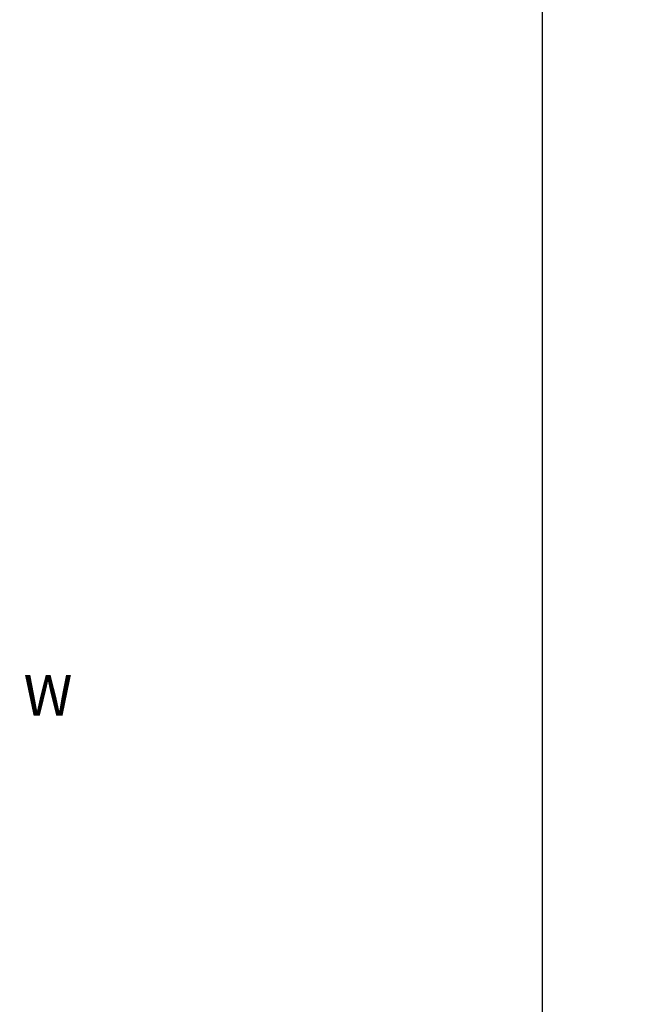
# Model space of a CAD drawing. Units: inches. Extents: x -77 to 516, y -119 to 536.
# Tile 5 of 11: x 378 to 468, y 15 to 159. Entities that reach past the tile are written whole.
import ezdxf

# ---------------------------------------------------------------- set-up
doc = ezdxf.new("R2010")
doc.units = ezdxf.units.IN
doc.header["$MEASUREMENT"] = 0
doc.layers.add('A-ANNO-DIMS', color=2, linetype='Continuous', lineweight=18)
doc.layers.add('text', color=170, linetype='Continuous', lineweight=18)
doc.styles.get("Standard").update_dxf_attribs({"font": 'arial.ttf'})
doc.dimstyles.get("Standard").update_dxf_attribs({"dimtxt": 12, "dimasz": 12, "dimexe": 0.18, "dimexo": 0.0625, "dimgap": 0.09, "dimtad": 0, "dimtih": 1, "dimtoh": 1, "dimdec": 1, "dimzin": 0, "dimdsep": 46, "dimlunit": 4, "dimtxsty": 'Standard', "dimcen": 0.09, "dimadec": 0, "dimazin": 0, "dimtfac": 1, "dimtdec": 1, "dimtofl": 0, "dimtmove": 0, "dimatfit": 3, "dimfxl": 1, "dimtolj": 1, "dimtzin": 0, "dimarcsym": 0})

# ---------------------------------------------------------------- blocks, each defined once
blk = doc.blocks.new('*D37')
at = {"layer": 'A-ANNO-DIMS', "color": 0, "lineweight": -2, "transparency": 16777216}
for p, q in [((373.81, 494.59), (454.58, 494.59)), ((454.4, 482.59), (454.4, 212.81)), ((454.4, -69.41), (454.4, 200.37)), ((309, -81.41), (454.58, -81.41))]:
    blk.add_line(p, q, dxfattribs=at)
at = {"layer": 'A-ANNO-DIMS', "color": 0, "transparency": 16777216}
for points in [[(452.4, 482.59), (456.4, 482.59), (454.4, 494.59)], [(452.4, -69.41), (456.4, -69.41), (454.4, -81.41)]]:
    blk.add_solid(points, dxfattribs=at)
at = {"layer": 'Defpoints', "color": 0, "transparency": 16777216}
for p in [(373.75, 494.59), (454.4, 494.59), (308.93, -81.41)]:
    blk.add_point(p, dxfattribs=at)
at = {"layer": 'A-ANNO-DIMS', "color": 0, "transparency": 16777216, "insert": (454.4, 206.59), "char_height": 12, "attachment_point": 5}
blk.add_mtext('\\A1;576', dxfattribs=at)

msp = doc.modelspace()

# ---------------------------------------------------------------- texts
at = {"layer": 'text', "insert": (378.1904, 62.941), "char_height": 6, "attachment_point": 1}
msp.add_mtext_dynamic_manual_height_columns('W', width=105.041962, gutter_width=1, heights=[0], dxfattribs=at)

# ---------------------------------------------------------------- dimensions: what is measured, and where the dimension line sits
at = {"layer": 'A-ANNO-DIMS'}
dim = msp.add_linear_dim(base=(454.4001, 494.5884), p1=(308.9336, -81.4116), p2=(373.7501, 494.5884), angle=90, dimstyle='Standard', override={"dimdec": 0, "dimlfac": 1, "dimrnd": 0, "dimzin": 0, "dimdsep": 46, "dimlunit": 2}, dxfattribs=at)
dim.commit()
dim.dimension.update_dxf_attribs({"geometry": '*D37', "text_midpoint": (454.4001, 206.5884)})

doc.saveas('drawing.dxf')
